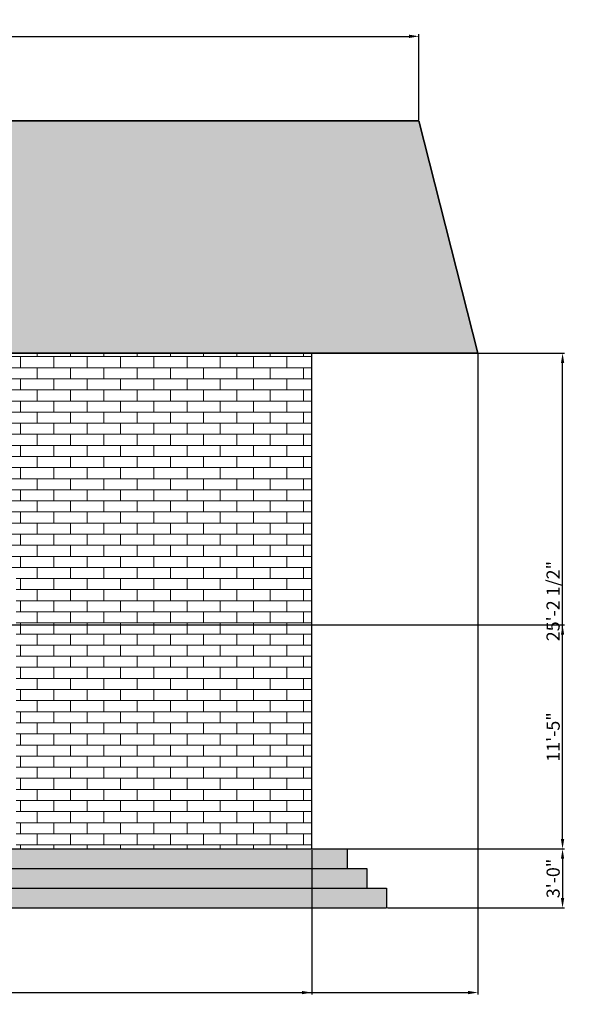
# Model space of a CAD drawing. Units: millimetres. Extents: x 1518 to 2850, y 936 to 2174.
# Tile 4 of 5: x 2336 to 2675, y 939 to 1540. Entities that reach past the tile are written whole.
import ezdxf

# ---------------------------------------------------------------- set-up
doc = ezdxf.new("R2010")
doc.units = ezdxf.units.MM
for name, color, linetype, lineweight, true_color in [('A-ANNO-DIMS', 9, 'Continuous', 18, 0xafd9aa), ('A-ELEV-BASE-PATT', 251, 'Continuous', 13, 0x636466), ('A-ELEV-WALL-PATT', 244, 'Continuous', 13, 0x991b1e), ('A-ROOF-PATT', 254, 'Continuous', 13, 0xfeeab9)]:
    doc.layers.add(name, color=color, linetype=linetype, lineweight=lineweight, true_color=true_color)
for name, color, linetype, lineweight in [('A-ELEV', 7, 'Continuous', 25), ('A-ELEV-BASE', 7, 'Continuous', 30), ('A-ROOF', 7, 'Continuous', 35)]:
    doc.layers.add(name, color=color, linetype=linetype, lineweight=lineweight)
doc.styles.get("Standard").update_dxf_attribs({"font": 'arial.ttf'})
doc.dimstyles.new('ISO-25', dxfattribs={"dimtxt": 8, "dimasz": 6, "dimexe": 1.25, "dimexo": 0.625, "dimtad": 1, "dimdec": 0, "dimlunit": 3, "dimtxsty": 'Standard', "dimcen": 2.5, "dimadec": 0, "dimazin": 0, "dimtfac": 1, "dimtdec": 0, "dimtmove": 0, "dimatfit": 3, "dimfxl": 1, "dimarcsym": 0})

# ---------------------------------------------------------------- blocks, each defined once
blk = doc.blocks.new('*D57')
at = {"layer": 'A-ANNO-DIMS', "color": 0, "lineweight": -2, "transparency": 16777216}
for p, q in [((1731.47, 1033.32), (1731.47, 945.05)), ((2514.61, 1033.32), (2514.61, 945.05)), ((1737.47, 946.3), (2508.61, 946.3))]:
    blk.add_line(p, q, dxfattribs=at)
at = {"layer": 'A-ANNO-DIMS', "color": 0, "transparency": 16777216}
for points in [[(1737.47, 947.3), (1737.47, 945.3), (1731.47, 946.3)], [(2508.61, 947.3), (2508.61, 945.3), (2514.61, 946.3)]]:
    blk.add_solid(points, dxfattribs=at)
at = {"layer": 'Defpoints', "color": 0, "transparency": 16777216}
for p in [(1731.47, 1033.95), (2514.61, 1033.95), (2514.61, 946.3)]:
    blk.add_point(p, dxfattribs=at)
at = {"layer": 'A-ANNO-DIMS', "color": 0, "transparency": 16777216, "insert": (2123.04, 951.01), "char_height": 8, "attachment_point": 5}
blk.add_mtext('65\'-3"', dxfattribs=at)
blk = doc.blocks.new('*D64')
at = {"layer": 'A-ANNO-DIMS', "color": 0, "lineweight": -2, "transparency": 16777216}
for p, q in [((2300.4, 1170.72), (2668.93, 1170.72)), ((2667.68, 1039.95), (2667.68, 1164.72)), ((2300.4, 1033.95), (2668.93, 1033.95))]:
    blk.add_line(p, q, dxfattribs=at)
at = {"layer": 'A-ANNO-DIMS', "color": 0, "transparency": 16777216}
for points in [[(2666.68, 1164.72), (2668.68, 1164.72), (2667.68, 1170.72)], [(2666.68, 1039.95), (2668.68, 1039.95), (2667.68, 1033.95)]]:
    blk.add_solid(points, dxfattribs=at)
at = {"layer": 'Defpoints', "color": 0, "transparency": 16777216}
for p in [(2299.77, 1170.72), (2667.68, 1170.72), (2299.77, 1033.95)]:
    blk.add_point(p, dxfattribs=at)
at = {"layer": 'A-ANNO-DIMS', "color": 0, "transparency": 16777216, "insert": (2662.97, 1102.33), "char_height": 8, "attachment_point": 5, "rotation": 90}
blk.add_mtext('11\'-5"', dxfattribs=at)
blk = doc.blocks.new('*D74')
at = {"layer": 'A-ANNO-DIMS', "color": 0, "lineweight": -2, "transparency": 16777216}
for p, q in [((1957.13, 1442.66), (1957.13, 1531.29)), ((1963.13, 1530.04), (2574.03, 1530.04)), ((2580.03, 1479.02), (2580.03, 1531.29))]:
    blk.add_line(p, q, dxfattribs=at)
at = {"layer": 'A-ANNO-DIMS', "color": 0, "transparency": 16777216}
for points in [[(1963.13, 1531.04), (1963.13, 1529.04), (1957.13, 1530.04)], [(2574.03, 1531.04), (2574.03, 1529.04), (2580.03, 1530.04)]]:
    blk.add_solid(points, dxfattribs=at)
at = {"layer": 'Defpoints', "color": 0, "transparency": 16777216}
for p in [(2580.03, 1530.04), (2580.03, 1478.39), (1957.13, 1442.04)]:
    blk.add_point(p, dxfattribs=at)
at = {"layer": 'A-ANNO-DIMS', "color": 0, "transparency": 16777216, "insert": (2268.58, 1534.75), "char_height": 8, "attachment_point": 5}
blk.add_mtext('51\'-11"', dxfattribs=at)
blk = doc.blocks.new('*D75')
at = {"layer": 'A-ANNO-DIMS', "color": 0, "lineweight": -2, "transparency": 16777216}
for p, q in [((2515.23, 1336.6), (2668.93, 1336.6)), ((2667.68, 1039.95), (2667.68, 1330.6)), ((2515.23, 1033.95), (2668.93, 1033.95))]:
    blk.add_line(p, q, dxfattribs=at)
at = {"layer": 'A-ANNO-DIMS', "color": 0, "transparency": 16777216}
for points in [[(2666.68, 1330.6), (2668.68, 1330.6), (2667.68, 1336.6)], [(2666.68, 1039.95), (2668.68, 1039.95), (2667.68, 1033.95)]]:
    blk.add_solid(points, dxfattribs=at)
at = {"layer": 'Defpoints', "color": 0, "transparency": 16777216}
for p in [(2514.61, 1336.6), (2667.68, 1336.6), (2514.61, 1033.95)]:
    blk.add_point(p, dxfattribs=at)
at = {"layer": 'A-ANNO-DIMS', "color": 0, "transparency": 16777216, "insert": (2662.92, 1185.27), "char_height": 8, "attachment_point": 5, "rotation": 90}
blk.add_mtext('25\'-2 1/2"', dxfattribs=at)
blk = doc.blocks.new('*D76')
at = {"layer": 'A-ANNO-DIMS', "color": 0, "lineweight": -2, "transparency": 16777216}
for p, q in [((2515.23, 1033.95), (2668.93, 1033.95)), ((2667.68, 1027.95), (2667.68, 1003.95)), ((2560.83, 997.95), (2668.93, 997.95))]:
    blk.add_line(p, q, dxfattribs=at)
at = {"layer": 'A-ANNO-DIMS', "color": 0, "transparency": 16777216}
for points in [[(2666.68, 1027.95), (2668.68, 1027.95), (2667.68, 1033.95)], [(2666.68, 1003.95), (2668.68, 1003.95), (2667.68, 997.95)]]:
    blk.add_solid(points, dxfattribs=at)
at = {"layer": 'Defpoints', "color": 0, "transparency": 16777216}
for p in [(2514.61, 1033.95), (2560.2, 997.95), (2667.68, 997.95)]:
    blk.add_point(p, dxfattribs=at)
at = {"layer": 'A-ANNO-DIMS', "color": 0, "transparency": 16777216, "insert": (2662.96, 1015.95), "char_height": 8, "attachment_point": 5, "rotation": 90}
blk.add_mtext('3\'-0"', dxfattribs=at)
blk = doc.blocks.new('*D77')
at = {"layer": 'A-ANNO-DIMS', "color": 0, "lineweight": -2, "transparency": 16777216}
for p, q in [((2616.03, 1335.98), (2616.03, 945.05)), ((1586.28, 997.32), (1586.28, 945.05)), ((1592.28, 946.3), (2610.03, 946.3))]:
    blk.add_line(p, q, dxfattribs=at)
at = {"layer": 'A-ANNO-DIMS', "color": 0, "transparency": 16777216}
for points in [[(1592.28, 947.3), (1592.28, 945.3), (1586.28, 946.3)], [(2610.03, 947.3), (2610.03, 945.3), (2616.03, 946.3)]]:
    blk.add_solid(points, dxfattribs=at)
at = {"layer": 'Defpoints', "color": 0, "transparency": 16777216}
for p in [(2616.03, 1336.6), (1586.28, 997.95), (2616.03, 946.3)]:
    blk.add_point(p, dxfattribs=at)
at = {"layer": 'A-ANNO-DIMS', "color": 0, "transparency": 16777216, "insert": (2101.15, 951.06), "char_height": 8, "attachment_point": 5}
blk.add_mtext('85\'-9 1/2"', dxfattribs=at)

msp = doc.modelspace()

# ---------------------------------------------------------------- hatches: boundary and pattern name
at = {"layer": 'A-ELEV-BASE-PATT'}
h = msp.add_hatch(dxfattribs=at)
h.set_pattern_fill('AR-SAND', color=256, scale=0.01, style=0)
h.paths.add_polyline_path([(2536.2, 1033.95), (1610.28, 1033.95), (1610.28, 1021.95), (1838.28, 1021.95), (2536.2, 1021.95)])
h.paths.add_polyline_path([(2548.2, 1021.95), (2536.2, 1021.95), (1838.28, 1021.95), (1598.28, 1021.95), (1598.28, 1009.95), (1826.28, 1009.95), (2548.2, 1009.95)])
h.paths.add_polyline_path([(2560.2, 1009.95), (2548.2, 1009.95), (1826.28, 1009.95), (1586.28, 1009.95), (1586.28, 997.95), (2560.2, 997.95)])
at = {"layer": 'A-ELEV-WALL-PATT'}
h = msp.add_hatch(dxfattribs=at)
h.set_pattern_fill('AR-BRSTD', color=256, scale=0.1)
h.paths.add_polyline_path([(1830.31, 1270.74), (1893.72, 1270.74), (1893.72, 1355.03), (1994.04, 1355.03), (1994.04, 1270.74), (2049.41, 1270.74), (2049.41, 1210.06), (2196.4, 1210.06), (2196.4, 1362.18), (2032.35, 1362.18), (2118.49, 1270.74), (2114.85, 1267.31), (1956.91, 1434.97), (1778.71, 1267.1), (1775.28, 1270.74), (1845.2, 1336.6), (1742.14, 1336.6), (1742.14, 1033.95), (1816.59, 1033.95), (1816.59, 1182.15), (1830.31, 1182.15)])
h.paths.add_polyline_path([(2120.6, 1234.32), (2120.6, 1333.95), (2128.33, 1333.95), (2128.33, 1234.32)], flags=16)
h.paths.add_polyline_path([(2139.93, 1234.32), (2139.93, 1333.95), (2147.66, 1333.95), (2147.66, 1234.32)], flags=16)
h.paths.add_polyline_path([(2160.03, 1234.32), (2160.03, 1333.95), (2167.76, 1333.95), (2167.76, 1234.32)], flags=16)
h.paths.add_polyline_path([(2514.61, 1336.6), (2302.13, 1336.6), (2302.13, 1256.02), (2317.67, 1256.02), (2317.67, 1275.95), (2326.9, 1275.95), (2326.9, 1210.06), (2326.9, 1199.48), (2334.04, 1199.48), (2334.04, 1033.95), (2514.61, 1033.95)])
h.paths.add_polyline_path([(2214.92, 1336.6), (2196.4, 1336.6), (2196.4, 1256.02), (2214.92, 1256.02)])
h.paths.add_polyline_path([(2205.44, 1170.72), (2299.77, 1170.72), (2299.77, 1033.95), (2326.9, 1033.95), (2326.9, 1199.48), (2326.9, 1210.06), (2317.67, 1210.06), (2049.41, 1210.06), (2049.41, 1033.95), (2205.44, 1033.95)])
h.paths.add_polyline_path([(2120.6, 1167.89), (2128.33, 1167.89), (2128.33, 1068.26), (2120.6, 1068.26)], flags=16)
h.paths.add_polyline_path([(2139.93, 1167.89), (2147.66, 1167.89), (2147.66, 1068.26), (2139.93, 1068.26)], flags=16)
h.paths.add_polyline_path([(2160.03, 1167.89), (2167.76, 1167.89), (2167.76, 1068.26), (2160.03, 1068.26)], flags=16)
h.paths.add_polyline_path([(1973.1, 1219.79), (1892.17, 1219.79), (1892.17, 1089.48), (1852.93, 1089.48), (1852.93, 1219.79), (1830.31, 1219.79), (1830.31, 1182.15), (1830.31, 1033.95), (1973.1, 1033.95)], flags=17)
at = {"layer": 'A-ROOF-PATT'}
h = msp.add_hatch(dxfattribs=at)
h.set_pattern_fill('AR-RROOF', color=256, scale=0.2)
h.paths.add_polyline_path([(1957.13, 1442.04), (2027.64, 1367.18), (2196.4, 1367.18), (2196.4, 1336.6), (2514.61, 1336.6), (2616.03, 1336.6), (2580.03, 1478.39), (1675.89, 1478.39), (1639.89, 1336.6), (1845.2, 1336.6)])

# ---------------------------------------------------------------- linework, layer by layer
at = {"layer": 'A-ELEV'}
msp.add_line((2514.61, 1033.95), (2514.61, 1336.6), dxfattribs=at)
at = {"layer": 'A-ELEV-BASE'}
for p, q in [((1610.28, 1033.95), (2536.2, 1033.95)), ((2536.2, 1033.95), (2536.2, 1021.95)), ((1838.28, 1021.95), (2536.2, 1021.95)), ((2536.2, 1021.95), (2548.2, 1021.95)), ((2548.2, 1021.95), (2548.2, 1009.95)), ((1826.28, 1009.95), (2548.2, 1009.95)), ((2548.2, 1009.95), (2560.2, 1009.95)), ((2560.2, 1009.95), (2560.2, 997.95)), ((1586.28, 997.95), (2560.2, 997.95))]:
    msp.add_line(p, q, dxfattribs=at)
at = {"layer": 'A-ROOF'}
for p, q in [((2580.03, 1478.39), (1675.89, 1478.39)), ((2580.03, 1478.39), (2616.03, 1336.6)), ((2514.61, 1336.6), (2196.4, 1336.6)), ((2514.61, 1336.6), (2616.03, 1336.6))]:
    msp.add_line(p, q, dxfattribs=at)

# ---------------------------------------------------------------- dimensions: what is measured, and where the dimension line sits
at = {"layer": 'A-ANNO-DIMS'}
for base, p1, p2, picture, middle in [((2580.03, 1530.04), (1957.13, 1442.04), (2580.03, 1478.39), '*D74', (2268.58, 1534.75)), ((2616.027, 946.2961), (1586.2782, 997.9461), (2616.027, 1336.6004), '*D77', (2101.1526, 951.0575)), ((2514.61, 946.3), (1731.47, 1033.95), (2514.61, 1033.95), '*D57', (2123.04, 951.01))]:
    dim = msp.add_linear_dim(base=base, p1=p1, p2=p2, dimstyle='ISO-25', override={"dimdec": 1, "dimlfac": 1, "dimrnd": 0, "dimzin": 1, "dimdsep": 46, "dimlunit": 4, "dimfrac": 2}, dxfattribs=at)
    dim.commit()
    dim.dimension.update_dxf_attribs({"geometry": picture, "text_midpoint": middle})
for base, p1, p2, picture, middle in [((2667.677, 1336.6004), (2514.6092, 1033.9461), (2514.6092, 1336.6004), '*D75', (2662.9156, 1185.2732)), ((2667.68, 1170.72), (2299.77, 1033.95), (2299.77, 1170.72), '*D64', (2662.97, 1102.33)), ((2667.68, 997.95), (2514.61, 1033.95), (2560.2, 997.95), '*D76', (2662.96, 1015.95))]:
    dim = msp.add_linear_dim(base=base, p1=p1, p2=p2, angle=90, dimstyle='ISO-25', override={"dimdec": 1, "dimlfac": 1, "dimrnd": 0, "dimzin": 1, "dimdsep": 46, "dimlunit": 4, "dimfrac": 2}, dxfattribs=at)
    dim.commit()
    dim.dimension.update_dxf_attribs({"geometry": picture, "text_midpoint": middle})

doc.saveas('drawing.dxf')
